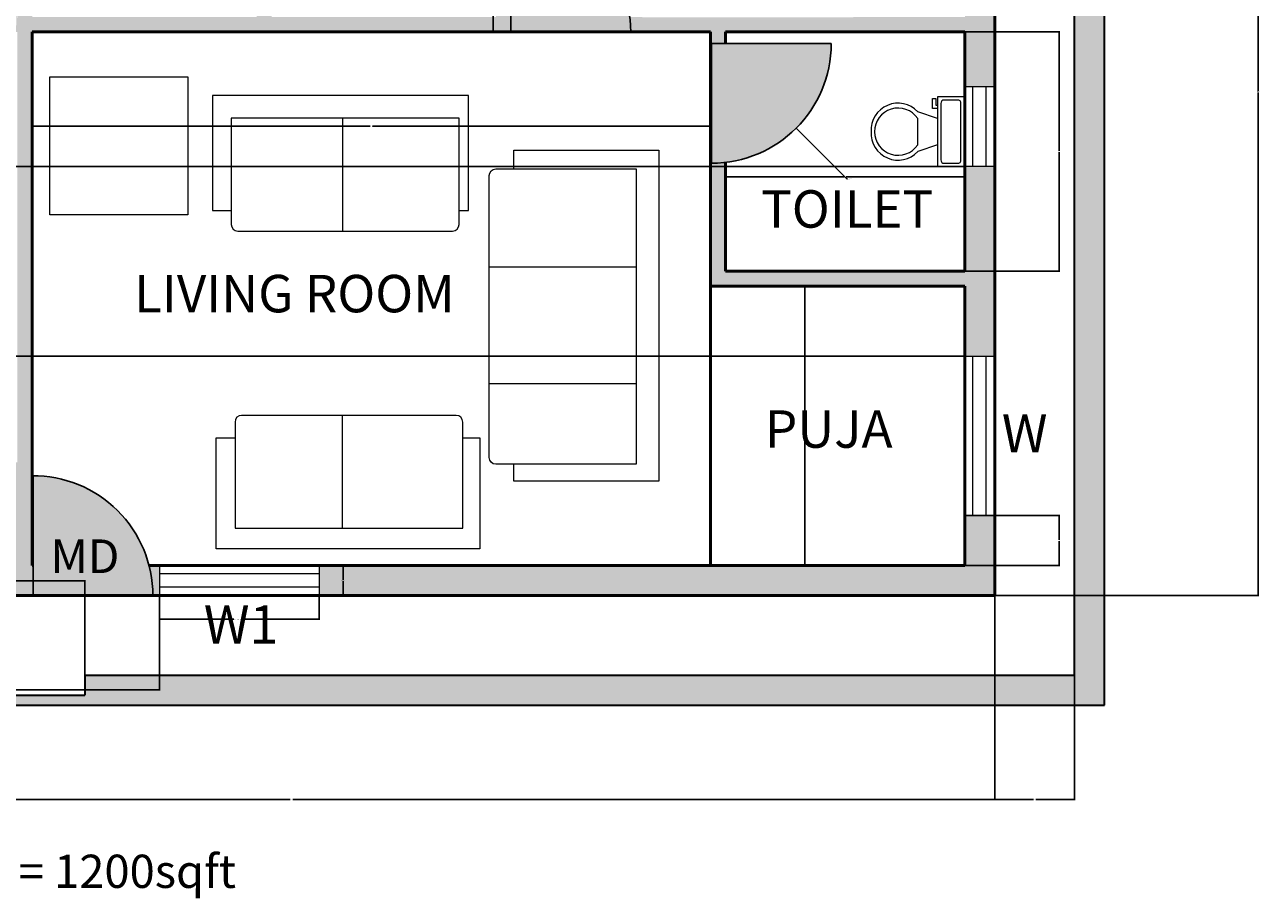
# Model space of a CAD drawing. Units: inches. Extents: x -48 to 546, y -53 to 467.
# Tile 2 of 3: x 174 to 546, y -53 to 210. Entities that reach past the tile are written whole.
import ezdxf

# ---------------------------------------------------------------- set-up
doc = ezdxf.new("R2010")
doc.units = ezdxf.units.IN
doc.header["$MEASUREMENT"] = 0
for name, color, linetype, lineweight in [('A-ANNO-DIMS', 2, 'Continuous', 18), ('A-ANNO-SYMB', 7, 'Continuous', 18), ('A-ANNO-TEXT', 7, 'Continuous', 18), ('A-AREA-IDEN', 7, 'Continuous', 25), ('A-DOOR', 4, 'Continuous', 25), ('A-FLOR-FIXT', 9, 'Continuous', 18), ('A-FURN', 8, 'Continuous', 18), ('A-GLAZ', 4, 'Continuous', 18), ('A-WALL', 7, 'Continuous', 50), ('C-PROP', 7, 'Continuous', 35)]:
    doc.layers.add(name, color=color, linetype=linetype, lineweight=lineweight)
for name, color, linetype, lineweight, true_color in [('A-FLOR-PATT', 253, 'Continuous', 13, 0x9898cc), ('A-WALL-PATT', 251, 'Continuous', 13, 0x636466), ('C-PROP-PATT', 251, 'Continuous', 13, 0x636466)]:
    doc.layers.add(name, color=color, linetype=linetype, lineweight=lineweight, true_color=true_color)
doc.styles.get("Standard").update_dxf_attribs({"font": 'arial.ttf'})
doc.dimstyles.get("Standard").update_dxf_attribs({"dimtxt": 0.18, "dimasz": 0.18, "dimexe": 0.18, "dimexo": 0.0625, "dimgap": 0.09, "dimtad": 0, "dimtih": 1, "dimtoh": 1, "dimdec": 4, "dimzin": 0, "dimdsep": 46, "dimtxsty": 'Standard', "dimcen": 0.09, "dimadec": 0, "dimazin": 0, "dimtfac": 1, "dimtdec": 4, "dimtofl": 0, "dimtmove": 0, "dimatfit": 3, "dimfxl": 1, "dimtolj": 1, "dimtzin": 0, "dimarcsym": 0})
picture_1 = doc.add_image_def('image1.png', size_in_pixel=(1024, 1024))

# ---------------------------------------------------------------- blocks, each defined once
blk = doc.blocks.new('*U2')
for p, q in [((9.5, -6), (9.5, -2)), ((-10, -8.5), (-8, -8.5)), ((-10, -9.5), (-10, -8.5)), ((-7, -9.5), (-10, -9.5)), ((-8, -8.5), (-8, -8)), ((-7, -8), (-7, -9.5)), ((-4, -8), (-6, -14)), ((4, -8), (6, -14)), ((4, -14), (-4, -14))]:
    blk.add_line(p, q)
blk.add_lwpolyline([(10.5, -8), (10.5, 0), (-10.5, 0), (-10.5, -8)], close=True)
for points in [[(-9.5, -2), (-9.5, -6)], [(8.5, -1), (-8.5, -1)], [(-8.5, -7), (8.5, -7)]]:
    blk.add_lwpolyline(points)
for centre, radius, start, end in [((-8.625, -1.875), 0.8839, 81.8699, 188.1301), ((8.625, -1.875), 0.8839, 351.8699, 98.1301), ((-8.625, -6.125), 0.8839, 171.869898, 278.1301), ((8.625, -6.125), 0.8839, 261.8699, 8.1301), ((-0.4772, -19.9188), 8.0953, 133.01722, 273.38), ((0.0374, -19.8731), 7.127, 124.50543, 269.7), ((-0.0373, -19.8731), 7.127, 270.3, 55.4946), ((0.4773, -19.9188), 8.0953, 266.62, 46.9828)]:
    blk.add_arc(centre, radius, start, end)
blk = doc.blocks.new('DOOR-SWING-36IN')
for p, q in [((0, 36), (0, 0)), ((0, 0), (36, 0))]:
    blk.add_line(p, q)
blk.add_arc((0, 0), 36, 0, 90)
blk = doc.blocks.new('VENT-24IN')
for p, q in [((0, 9), (0, 0)), ((24, 9), (24, 0)), ((0, 6.5), (24, 6.5)), ((0, 2.5), (24, 2.5))]:
    blk.add_line(p, q)
blk = doc.blocks.new('WIN-48IN-FRONT')
for p, q in [((0, 9), (0, 0)), ((48, 9), (48, 0)), ((48, 6.49), (0, 6.49)), ((48, 2.49), (0, 2.49)), ((48, 2.49), (0, 2.49)), ((48, 2.49), (0, 2.49))]:
    blk.add_line(p, q)
blk = doc.blocks.new('*D14')
at = {"layer": 'A-ANNO-DIMS', "color": 0, "lineweight": -2, "transparency": 16777216}
for p, q in [((320.64, 244.01), (315.12, 244.01)), ((315.3, 243.83), (315.3, 226.2)), ((315.3, 208.19), (315.3, 225.83)), ((320.64, 208.01), (315.12, 208.01))]:
    blk.add_line(p, q, dxfattribs=at)
at = {"layer": 'A-ANNO-DIMS', "color": 0, "transparency": 16777216}
for points in [[(315.27, 243.83), (315.33, 243.83), (315.3, 244.01)], [(315.27, 208.19), (315.33, 208.19), (315.3, 208.01)]]:
    blk.add_solid(points, dxfattribs=at)
at = {"layer": 'Defpoints', "color": 0, "transparency": 16777216}
for p in [(315.3, 244.01), (320.7, 244.01), (320.7, 208.01)]:
    blk.add_point(p, dxfattribs=at)
at = {"layer": 'A-ANNO-DIMS', "color": 0, "transparency": 16777216, "insert": (315.3, 226.01), "char_height": 0.18, "attachment_point": 5}
blk.add_mtext('\\A1;DOOR 3\'-0" TYP.', dxfattribs=at)
blk = doc.blocks.new('*D18')
at = {"layer": 'A-ANNO-DIMS', "color": 0, "lineweight": -2, "transparency": 16777216}
for p, q in [((215, 38.45), (215, 31.13)), ((263, 38.45), (263, 31.13)), ((215.18, 31.31), (237.31, 31.31)), ((262.82, 31.31), (240.69, 31.31))]:
    blk.add_line(p, q, dxfattribs=at)
at = {"layer": 'A-ANNO-DIMS', "color": 0, "transparency": 16777216}
for points in [[(215.18, 31.34), (215.18, 31.28), (215, 31.31)], [(262.82, 31.34), (262.82, 31.28), (263, 31.31)]]:
    blk.add_solid(points, dxfattribs=at)
at = {"layer": 'Defpoints', "color": 0, "transparency": 16777216}
for p in [(215, 38.51), (263, 38.51), (263, 31.31)]:
    blk.add_point(p, dxfattribs=at)
at = {"layer": 'A-ANNO-DIMS', "color": 0, "transparency": 16777216, "insert": (239, 31.31), "char_height": 0.18, "attachment_point": 5}
blk.add_mtext('\\A1;FRONT WINDOW 4\'-0" TYP.', dxfattribs=at)
blk = doc.blocks.new('*D19')
at = {"layer": 'A-ANNO-DIMS', "color": 0, "lineweight": -2, "transparency": 16777216}
for p, q in [((263.06, 47.51), (270.38, 47.51)), ((270.2, 47.33), (270.2, 43.2)), ((270.2, 38.69), (270.2, 42.83)), ((263.06, 38.51), (270.38, 38.51))]:
    blk.add_line(p, q, dxfattribs=at)
at = {"layer": 'A-ANNO-DIMS', "color": 0, "transparency": 16777216}
for points in [[(270.17, 47.33), (270.23, 47.33), (270.2, 47.51)], [(270.17, 38.69), (270.23, 38.69), (270.2, 38.51)]]:
    blk.add_solid(points, dxfattribs=at)
at = {"layer": 'Defpoints', "color": 0, "transparency": 16777216}
for p in [(263, 47.51), (270.2, 47.51), (263, 38.51)]:
    blk.add_point(p, dxfattribs=at)
at = {"layer": 'A-ANNO-DIMS', "color": 0, "transparency": 16777216, "insert": (270.2, 43.01), "char_height": 0.18, "attachment_point": 5}
blk.add_mtext('\\A1;0\'-9" TYP.', dxfattribs=at)
blk = doc.blocks.new('*D26')
at = {"layer": 'A-ANNO-DIMS', "color": 0, "lineweight": -2, "transparency": 16777216}
for p, q in [((43.2, 38.45), (43.2, -23.08)), ((466.2, 38.45), (466.2, -23.08)), ((43.38, -22.9), (254.3, -22.9)), ((466.02, -22.9), (255.1, -22.9))]:
    blk.add_line(p, q, dxfattribs=at)
at = {"layer": 'A-ANNO-DIMS', "color": 0, "transparency": 16777216}
for points in [[(43.38, -22.87), (43.38, -22.93), (43.2, -22.9)], [(466.02, -22.87), (466.02, -22.93), (466.2, -22.9)]]:
    blk.add_solid(points, dxfattribs=at)
at = {"layer": 'Defpoints', "color": 0, "transparency": 16777216}
for p in [(43.2, 38.51), (466.2, 38.51), (466.2, -22.9)]:
    blk.add_point(p, dxfattribs=at)
at = {"layer": 'A-ANNO-DIMS', "color": 0, "transparency": 16777216, "insert": (254.7, -22.9), "char_height": 0.18, "attachment_point": 5}
blk.add_mtext('\\A1;35\'-3"', dxfattribs=at)
blk = doc.blocks.new('*D27')
at = {"layer": 'A-ANNO-DIMS', "color": 0, "lineweight": -2, "transparency": 16777216}
for p, q in [((466.26, 341.51), (545.59, 341.51)), ((545.41, 341.33), (545.41, 190.2)), ((545.41, 38.69), (545.41, 189.83)), ((466.26, 38.51), (545.59, 38.51))]:
    blk.add_line(p, q, dxfattribs=at)
at = {"layer": 'A-ANNO-DIMS', "color": 0, "transparency": 16777216}
for points in [[(545.38, 341.33), (545.44, 341.33), (545.41, 341.51)], [(545.38, 38.69), (545.44, 38.69), (545.41, 38.51)]]:
    blk.add_solid(points, dxfattribs=at)
at = {"layer": 'Defpoints', "color": 0, "transparency": 16777216}
for p in [(466.2, 341.51), (545.41, 341.51), (466.2, 38.51)]:
    blk.add_point(p, dxfattribs=at)
at = {"layer": 'A-ANNO-DIMS', "color": 0, "transparency": 16777216, "insert": (545.41, 190.01), "char_height": 0.18, "attachment_point": 5}
blk.add_mtext('\\A1;25\'-3"', dxfattribs=at)
blk = doc.blocks.new('*D28')
at = {"layer": 'A-ANNO-DIMS', "color": 0, "lineweight": -2, "transparency": 16777216}
for p, q in [((466.2, 38.45), (466.2, -23.08)), ((490.2, 14.45), (490.2, -23.08)), ((466.38, -22.9), (477.87, -22.9)), ((490.02, -22.9), (478.53, -22.9))]:
    blk.add_line(p, q, dxfattribs=at)
at = {"layer": 'A-ANNO-DIMS', "color": 0, "transparency": 16777216}
for points in [[(466.38, -22.87), (466.38, -22.93), (466.2, -22.9)], [(490.02, -22.87), (490.02, -22.93), (490.2, -22.9)]]:
    blk.add_solid(points, dxfattribs=at)
at = {"layer": 'Defpoints', "color": 0, "transparency": 16777216}
for p in [(466.2, 38.51), (490.2, 14.51), (490.2, -22.9)]:
    blk.add_point(p, dxfattribs=at)
at = {"layer": 'A-ANNO-DIMS', "color": 0, "transparency": 16777216, "insert": (478.2, -22.9), "char_height": 0.18, "attachment_point": 5}
blk.add_mtext('\\A1;2\'-0"', dxfattribs=at)
blk = doc.blocks.new('*D36')
at = {"layer": 'A-ANNO-DIMS', "color": 0, "lineweight": -2, "transparency": 16777216}
for p, q in [((176.7, 207.95), (176.7, 179.43)), ((380.7, 207.95), (380.7, 179.43)), ((176.88, 179.61), (278.31, 179.61)), ((380.52, 179.61), (279.09, 179.61))]:
    blk.add_line(p, q, dxfattribs=at)
at = {"layer": 'A-ANNO-DIMS', "color": 0, "transparency": 16777216}
for points in [[(176.88, 179.64), (176.88, 179.58), (176.7, 179.61)], [(380.52, 179.64), (380.52, 179.58), (380.7, 179.61)]]:
    blk.add_solid(points, dxfattribs=at)
at = {"layer": 'Defpoints', "color": 0, "transparency": 16777216}
for p in [(176.7, 208.01), (380.7, 208.01), (176.7, 179.61)]:
    blk.add_point(p, dxfattribs=at)
at = {"layer": 'A-ANNO-DIMS', "color": 0, "transparency": 16777216, "insert": (278.7, 179.61), "char_height": 0.18, "attachment_point": 5}
blk.add_mtext('\\A1;17\'-0"', dxfattribs=at)
blk = doc.blocks.new('*D37')
at = {"layer": 'A-ANNO-DIMS', "color": 0, "lineweight": -2, "transparency": 16777216}
for p, q in [((385.2, 136.08), (385.2, 164.59)), ((385.38, 164.41), (420.87, 164.41)), ((457.02, 164.41), (421.53, 164.41)), ((457.2, 136.08), (457.2, 164.59))]:
    blk.add_line(p, q, dxfattribs=at)
at = {"layer": 'A-ANNO-DIMS', "color": 0, "transparency": 16777216}
for points in [[(385.38, 164.44), (385.38, 164.38), (385.2, 164.41)], [(457.02, 164.44), (457.02, 164.38), (457.2, 164.41)]]:
    blk.add_solid(points, dxfattribs=at)
at = {"layer": 'Defpoints', "color": 0, "transparency": 16777216}
for p in [(457.2, 164.41), (385.2, 136.01), (457.2, 136.01)]:
    blk.add_point(p, dxfattribs=at)
at = {"layer": 'A-ANNO-DIMS', "color": 0, "transparency": 16777216, "insert": (421.2, 164.41), "char_height": 0.18, "attachment_point": 5}
blk.add_mtext('\\A1;6\'-0"', dxfattribs=at)
blk = doc.blocks.new('*D38')
at = {"layer": 'A-ANNO-DIMS', "color": 0, "lineweight": -2, "transparency": 16777216}
for p, q in [((457.26, 208.01), (485.78, 208.01)), ((485.6, 207.83), (485.6, 172.2)), ((485.6, 136.19), (485.6, 171.83)), ((457.26, 136.01), (485.78, 136.01))]:
    blk.add_line(p, q, dxfattribs=at)
at = {"layer": 'A-ANNO-DIMS', "color": 0, "transparency": 16777216}
for points in [[(485.57, 207.83), (485.63, 207.83), (485.6, 208.01)], [(485.57, 136.19), (485.63, 136.19), (485.6, 136.01)]]:
    blk.add_solid(points, dxfattribs=at)
at = {"layer": 'Defpoints', "color": 0, "transparency": 16777216}
for p in [(457.2, 208.01), (457.2, 136.01), (485.6, 136.01)]:
    blk.add_point(p, dxfattribs=at)
at = {"layer": 'A-ANNO-DIMS', "color": 0, "transparency": 16777216, "insert": (485.6, 172.01), "char_height": 0.18, "attachment_point": 5}
blk.add_mtext('\\A1;6\'-0"', dxfattribs=at)
blk = doc.blocks.new('*D39')
at = {"layer": 'A-ANNO-DIMS', "color": 0, "lineweight": -2, "transparency": 16777216}
for p, q in [((380.76, 131.51), (409.28, 131.51)), ((409.1, 131.33), (409.1, 89.7)), ((409.1, 47.69), (409.1, 89.33)), ((380.76, 47.51), (409.28, 47.51))]:
    blk.add_line(p, q, dxfattribs=at)
at = {"layer": 'A-ANNO-DIMS', "color": 0, "transparency": 16777216}
for points in [[(409.07, 131.33), (409.13, 131.33), (409.1, 131.51)], [(409.07, 47.69), (409.13, 47.69), (409.1, 47.51)]]:
    blk.add_solid(points, dxfattribs=at)
at = {"layer": 'Defpoints', "color": 0, "transparency": 16777216}
for p in [(380.7, 131.51), (380.7, 47.51), (409.1, 47.51)]:
    blk.add_point(p, dxfattribs=at)
at = {"layer": 'A-ANNO-DIMS', "color": 0, "transparency": 16777216, "insert": (409.1, 89.51), "char_height": 0.18, "attachment_point": 5}
blk.add_mtext('\\A1;7\'-0"', dxfattribs=at)
blk = doc.blocks.new('*D41')
at = {"layer": 'A-ANNO-DIMS', "color": 0, "lineweight": -2, "transparency": 16777216}
for p, q in [((120, 38.45), (120, 9.93)), ((215, 38.45), (215, 9.93)), ((120.18, 10.11), (167.1, 10.11)), ((214.82, 10.11), (167.9, 10.11))]:
    blk.add_line(p, q, dxfattribs=at)
at = {"layer": 'A-ANNO-DIMS', "color": 0, "transparency": 16777216}
for points in [[(120.18, 10.14), (120.18, 10.08), (120, 10.11)], [(214.82, 10.14), (214.82, 10.08), (215, 10.11)]]:
    blk.add_solid(points, dxfattribs=at)
at = {"layer": 'Defpoints', "color": 0, "transparency": 16777216}
for p in [(120, 38.51), (215, 38.51), (120, 10.11)]:
    blk.add_point(p, dxfattribs=at)
at = {"layer": 'A-ANNO-DIMS', "color": 0, "transparency": 16777216, "insert": (167.5, 10.11), "char_height": 0.18, "attachment_point": 5}
blk.add_mtext('\\A1;7\'-11"', dxfattribs=at)
blk = doc.blocks.new('*D44')
at = {"layer": 'A-ANNO-DIMS', "color": 0, "lineweight": -2, "transparency": 16777216}
for p, q in [((457.26, 62.5), (485.78, 62.5)), ((485.6, 62.32), (485.6, 55.19)), ((485.6, 47.69), (485.6, 54.82)), ((457.26, 47.51), (485.78, 47.51))]:
    blk.add_line(p, q, dxfattribs=at)
at = {"layer": 'A-ANNO-DIMS', "color": 0, "transparency": 16777216}
for points in [[(485.57, 62.32), (485.63, 62.32), (485.6, 62.5)], [(485.57, 47.69), (485.63, 47.69), (485.6, 47.51)]]:
    blk.add_solid(points, dxfattribs=at)
at = {"layer": 'Defpoints', "color": 0, "transparency": 16777216}
for p in [(457.2, 62.5), (457.2, 47.51), (485.6, 47.51)]:
    blk.add_point(p, dxfattribs=at)
at = {"layer": 'A-ANNO-DIMS', "color": 0, "transparency": 16777216, "insert": (485.6, 55.01), "char_height": 0.18, "attachment_point": 5}
blk.add_mtext('\\A1;1\'-3"', dxfattribs=at)
blk = doc.blocks.new('*D45')
at = {"layer": 'A-ANNO-DIMS', "color": 0, "lineweight": -2, "transparency": 16777216}
for p, q in [((456.95, 167.5), (-18.38, 167.5)), ((-18.2, 167.32), (-18.2, 139.18)), ((-18.2, 110.68), (-18.2, 138.82)), ((457.14, 110.5), (-18.38, 110.5))]:
    blk.add_line(p, q, dxfattribs=at)
at = {"layer": 'A-ANNO-DIMS', "color": 0, "transparency": 16777216}
for points in [[(-18.23, 167.32), (-18.17, 167.32), (-18.2, 167.5)], [(-18.23, 110.68), (-18.17, 110.68), (-18.2, 110.5)]]:
    blk.add_solid(points, dxfattribs=at)
at = {"layer": 'Defpoints', "color": 0, "transparency": 16777216}
for p in [(457.01, 167.5), (-18.2, 110.5), (457.2, 110.5)]:
    blk.add_point(p, dxfattribs=at)
at = {"layer": 'A-ANNO-DIMS', "color": 0, "transparency": 16777216, "insert": (-18.2, 139), "char_height": 0.18, "attachment_point": 5}
blk.add_mtext('\\A1;4\'-9"', dxfattribs=at)
blk = doc.blocks.new('*D49')
at = {"layer": 'A-ANNO-DIMS', "color": 0, "lineweight": -2, "transparency": 16777216}
for p, q in [((103, 14.58), (103, 43.09)), ((103.18, 42.91), (147.21, 42.91)), ((192.32, 42.91), (148.29, 42.91)), ((192.5, 14.58), (192.5, 43.09))]:
    blk.add_line(p, q, dxfattribs=at)
at = {"layer": 'A-ANNO-DIMS', "color": 0, "transparency": 16777216}
for points in [[(103.18, 42.94), (103.18, 42.88), (103, 42.91)], [(192.32, 42.94), (192.32, 42.88), (192.5, 42.91)]]:
    blk.add_solid(points, dxfattribs=at)
at = {"layer": 'Defpoints', "color": 0, "transparency": 16777216}
for p in [(192.5, 42.91), (103, 14.51), (192.5, 14.51)]:
    blk.add_point(p, dxfattribs=at)
at = {"layer": 'A-ANNO-DIMS', "color": 0, "transparency": 16777216, "insert": (147.75, 42.91), "char_height": 0.18, "attachment_point": 5}
blk.add_mtext('\\A1;7\'-5 1/2"', dxfattribs=at)
blk = doc.blocks.new('*D51')
at = {"layer": 'A-ANNO-DIMS', "color": 0, "lineweight": -2, "transparency": 16777216}
for p, q in [((380.91, 204.5), (381.09, 204.5)), ((381, 204.41), (381, 204.59)), ((421.73, 163.77), (406.58, 178.92)), ((421.91, 163.77), (421.73, 163.77))]:
    blk.add_line(p, q, dxfattribs=at)
at = {"layer": 'A-ANNO-DIMS', "color": 0, "transparency": 16777216}
blk.add_solid([(406.6, 178.94), (406.56, 178.9), (406.46, 179.04)], dxfattribs=at)
at = {"layer": 'Defpoints', "color": 0, "transparency": 16777216}
for p in [(381, 204.5), (406.46, 179.04)]:
    blk.add_point(p, dxfattribs=at)
at = {"layer": 'A-ANNO-DIMS', "color": 0, "transparency": 16777216, "insert": (422.52, 163.77), "char_height": 0.18, "attachment_point": 5}
blk.add_mtext('\\A1;6X R3\'-0"', dxfattribs=at)

msp = doc.modelspace()

# ---------------------------------------------------------------- hatches: boundary and pattern name
at = {"layer": 'A-FLOR-PATT'}
h = msp.add_hatch(color=256, dxfattribs=at)
h.dxf.hatch_style = 1
h.paths.add_polyline_path([(208.19994, 330.01344), (172.19994, 330.01344), (172.19994, 294.01344, 0.414213549)])
h.paths.add_polyline_path([(320.5, 332.5), (284.5, 332.5, 0.414213562), (320.5, 296.5)])
h.paths.add_polyline_path([(417, 204.5), (381, 204.5), (381, 168.5, 0.414213562)])
h.paths.add_polyline_path([(177, 74.5), (177, 38.51344), (213, 38.51344, 0.414104244)])
h.paths.add_polyline_path([(172, 244, 0.414104258), (136, 208.01344), (172, 208.01344)])
h.paths.add_polyline_path([(320.69994, 244.01344), (320.69994, 212.51344), (320.69994, 208.01344), (356.69994, 208.01344, 0.414213532)])
h.paths.add_polyline_path([(172.19994, 78.5), (52.19994, 78.5), (52.19994, 47.51344), (172.19994, 47.51344)])
h.paths.add_polyline_path([(126, 74), (166, 74), (166, 54.5), (126, 54.5)], flags=16)
h.paths.add_polyline_path([(101, 53), (56.5, 53), (56.5, 74.5), (101, 74.5)], flags=16)
h.paths.add_polyline_path([(141, 69), (162.5, 69), (162.5, 58.5), (141, 58.5)], flags=0)
h.paths.add_polyline_path([(97.5, 55), (83, 55), (83, 67.5), (97.5, 67.5)], flags=0)
h.paths.add_polyline_path([(84, 61.5, -1), (96, 61.5, -1)], flags=0)
h.paths.add_polyline_path([(88.5, 71.5, -1), (92.5, 71.5, -1)], flags=0)
h.paths.add_polyline_path([(90, 71.5, -1), (91, 71.5, -1)], flags=0)
h.paths.add_polyline_path([(162, 64.5, -1), (158, 64.5, -1)], flags=0)
h.paths.add_polyline_path([(75, 55), (60.5, 55), (60.5, 67.5), (75, 67.5)], flags=0)
h.paths.add_polyline_path([(61.5, 61.5, -1), (73.5, 61.5, -1)], flags=0)
h.paths.add_polyline_path([(66, 71.5, -1), (70, 71.5, -1)], flags=0)
h.paths.add_polyline_path([(67.5, 71.5, -1), (68.5, 71.5, -1)], flags=0)
h.paths.add_polyline_path([(176.42827, 40.63764), (207.16292, 40.63764), (207.16292, 57.88764), (176.42827, 57.88764)], flags=9)
h = msp.add_hatch(color=256, dxfattribs=at)
h.dxf.hatch_style = 1
h.paths.add_polyline_path([(177, 74.5), (177, 38.51344), (213, 38.51344, 0.414104244)])
at = {"layer": 'A-WALL-PATT'}
h = msp.add_hatch(color=256, dxfattribs=at)
h.dxf.hatch_style = 1
h.paths.add_polyline_path([(282.44994, 341.51344), (234.44994, 341.51344), (234.44994, 332.51344), (244.19994, 332.51344), (244.19994, 212.51344), (176.69994, 212.51344), (176.69994, 294.29579, -0.031342215), (172.19994, 294.01344), (172.19994, 212.51344), (172.00059, 208.01344), (172.19994, 208.01344), (172.19994, 47.51344), (120, 47.51344), (120, 38.51344), (177, 38.51344), (177, 47.51344), (176.69994, 47.51344), (176.69994, 208.01344), (320.69994, 208.01344), (320.69994, 244.01344), (320.69994, 296.50056, -0.031331714), (316.19994, 296.75774), (316.19994, 212.51344), (248.69994, 212.51344), (248.69994, 332.51344), (282.44994, 332.51344)])
h.paths.add_polyline_path([(466.19994, 341.51344), (306.44994, 341.51344), (306.44994, 332.51344), (316.19994, 332.51344), (457.19994, 332.51344), (457.19994, 304.5), (466.19994, 304.5)])
h.paths.add_polyline_path([(466.19994, 256.5), (457.19994, 256.5), (457.19994, 212.51344), (423.64319, 212.51344), (423.64319, 212.34928), (365.34701, 212.34928), (356.41758, 212.51344, -0.031342215), (356.69994, 208.01344), (380.69994, 208.01344), (380.69994, 204.5), (385.19994, 204.5), (385.19994, 208.01344), (457.19994, 208.01344), (457.19994, 191.5), (466.19994, 191.5)])
h.paths.add_polyline_path([(210.44994, 341.51344), (43.19994, 341.51344), (43.19994, 303.5), (52.19994, 303.5), (52.19994, 332.51344), (172.19994, 332.51344), (172.19994, 330.01344), (176.69994, 330.01344), (176.69994, 332.51344), (210.44994, 332.51344)])
h.paths.add_polyline_path([(52.19994, 208.01344), (136, 208.01344, -0.031342955), (136.28405, 212.51344), (52.19994, 212.51344), (52.19994, 255.5), (43.19994, 255.5), (43.19994, 38.51344), (72, 38.51344), (72, 47.51344), (52.19994, 47.51344)])
h.paths.add_polyline_path([(466.19994, 62.5), (457.19994, 62.5), (457.19994, 47.51344), (380.69994, 47.51344), (263, 47.51344), (263, 38.51344), (466.19994, 38.51344)])
h.paths.add_polyline_path([(215, 47.51344), (211.85338, 47.51344, -0.063257301), (213, 38.51344), (215, 38.51344)])
h.paths.add_polyline_path([(466.19994, 167.5), (457.19994, 167.5), (457.19994, 136.01344), (385.19994, 136.01344), (385.19994, 168.74583, -0.031326837), (380.69994, 168.50125), (380.69994, 131.51344), (457.19994, 131.51344), (457.19994, 110.5), (466.19994, 110.5)])
h = msp.add_hatch(color=256, dxfattribs=at)
h.dxf.hatch_style = 1
h.paths.add_polyline_path([(210.44994, 341.51344), (43.19994, 341.51344), (43.19994, 303.5), (52.19994, 303.5), (52.19994, 332.51344), (172.19994, 332.51344), (172.19994, 330.01344), (176.69994, 330.01344), (176.69994, 332.51344), (210.44994, 332.51344)])
h.paths.add_polyline_path([(466.19994, 341.51344), (306.44994, 341.51344), (306.44994, 332.51344), (316.19994, 332.51344), (457.19994, 332.51344), (457.19994, 304.5), (466.19994, 304.5)])
h.paths.add_polyline_path([(282.44994, 341.51344), (234.44994, 341.51344), (234.44994, 332.51344), (244.19994, 332.51344), (244.19994, 212.51344), (176.69994, 212.51344), (176.69994, 294.29579, -0.031342215), (172.19994, 294.01344), (172.19994, 212.51344), (172.00059, 208.01344), (172.19994, 208.01344), (172.19994, 47.51344), (120, 47.51344), (120, 38.51344), (177, 38.51344), (177, 47.51344), (176.69994, 47.51344), (176.69994, 208.01344), (320.69994, 208.01344), (320.69994, 244.01344), (320.69994, 296.50056, -0.031331714), (316.19994, 296.75774), (316.19994, 212.51344), (248.69994, 212.51344), (248.69994, 332.51344), (282.44994, 332.51344)])
h.paths.add_polyline_path([(52.19994, 255.5), (43.19994, 255.5), (43.19994, 38.51344), (72, 38.51344), (72, 47.51344), (52.19994, 47.51344), (52.19994, 208.01344), (136, 208.01344, -0.031342955), (136.28405, 212.51344), (52.19994, 212.51344)])
h.paths.add_polyline_path([(466.19994, 256.5), (457.19994, 256.5), (457.19994, 212.51344), (423.64319, 212.51344), (423.64319, 212.34928), (365.34701, 212.34928), (356.41758, 212.51344, -0.031342215), (356.69994, 208.01344), (380.69994, 208.01344), (380.69994, 204.5), (385.19994, 204.5), (385.19994, 208.01344), (457.19994, 208.01344), (457.19994, 191.5), (466.19994, 191.5)])
h.paths.add_polyline_path([(466.19994, 167.5), (457.19994, 167.5), (457.19994, 136.01344), (385.19994, 136.01344), (385.19994, 168.74583, -0.031326837), (380.69994, 168.50125), (380.69994, 131.51344), (457.19994, 131.51344), (457.19994, 110.5), (466.19994, 110.5)])
h.paths.add_polyline_path([(466.19994, 62.5), (457.19994, 62.5), (457.19994, 47.51344), (380.69994, 47.51344), (263, 47.51344), (263, 38.51344), (466.19994, 38.51344)])
h.paths.add_polyline_path([(215, 47.51344), (211.85338, 47.51344, -0.063257301), (213, 38.51344), (215, 38.51344)])
at = {"layer": 'C-PROP-PATT'}
h = msp.add_hatch(color=256, dxfattribs=at)
h.dxf.hatch_style = 1
h.paths.add_polyline_path([(499.19994, 374.51344), (10.19994, 374.51344), (10.19994, 5.51344), (103, 5.51344), (103, 14.51344), (19.19994, 14.51344), (19.19994, 365.51344), (490.19994, 365.51344), (490.19994, 14.51344), (192.5, 14.51344), (192.5, 5.51344), (499.19994, 5.51344)])
h = msp.add_hatch(color=256, dxfattribs=at)
h.dxf.hatch_style = 1
h.paths.add_polyline_path([(192.5, 8.5), (103, 8.5), (103, 5.5), (192.5, 5.5)])

# ---------------------------------------------------------------- linework, layer by layer
at = {"layer": 'A-DOOR'}
for p, q in [((417, 204.5), (380.69994, 204.5)), ((381, 204.5), (381, 168.5)), ((177, 74.5), (177, 38.5)), ((177, 38.5), (213, 38.5))]:
    msp.add_line(p, q, dxfattribs=at)
for centre, start, end in [((381, 204.5), 270, 0), ((177, 38.5), 0, 90.4775597)]:
    msp.add_arc(centre, 36, start, end, dxfattribs=at)
at = {"layer": 'A-FURN'}
for p, q in [((269.97917, 182.0553), (269.97917, 148.07718)), ((314.08115, 137.36171), (358.24372, 137.36171)), ((314.08115, 102.29131), (358.24372, 102.29131)), ((269.97455, 92.72533), (269.97455, 58.6555))]:
    msp.add_line(p, q, dxfattribs=at)
for points in [[(305.09029, 154.33241), (307.92183, 154.33241), (307.92183, 188.84458), (230.9039, 188.84458), (230.9039, 154.33241), (236.56698, 154.33241)], [(321.51323, 166.77943), (321.51323, 172.43716), (365.11896, 172.43716), (365.11896, 72.86107), (321.51323, 72.86107), (321.51323, 77.95303)], [(306.2229, 85.87385), (311.31968, 85.87385), (311.31968, 52.49324), (232.03652, 52.49324), (232.03652, 85.87385), (237.6996, 85.87385)]]:
    msp.add_lwpolyline(points, dxfattribs=at)
for points in [[(238.56698, 148.10891), (303.09029, 148.10891, 0.414213562), (305.09029, 150.10891), (305.09029, 182.0553), (236.56698, 182.0553), (236.56698, 150.10891, 0.414213562)], [(316.15122, 166.77943), (358.32326, 166.77943), (358.32326, 77.95303), (316.15122, 77.95303, -0.414213562), (314.15122, 79.95303), (314.15122, 164.77943, -0.414213562)], [(237.6996, 58.71674), (306.2229, 58.71674), (306.2229, 90.66313, 0.414213562), (304.2229, 92.66313), (239.6996, 92.66313, 0.414213562), (237.6996, 90.66313)]]:
    msp.add_lwpolyline(points, format="xyb", close=True, dxfattribs=at)
at = {"layer": 'A-GLAZ'}
for p, q in [((457.19994, 110.5), (466.19994, 110.5)), ((459.50001, 110.5), (459.50001, 62.5)), ((463.50001, 110.5), (463.50001, 62.5)), ((463.50001, 110.5), (463.50001, 62.5)), ((463.50001, 110.5), (463.50001, 62.5)), ((457.19994, 62.5), (466.19994, 62.5))]:
    msp.add_line(p, q, dxfattribs=at)
at = {"layer": 'A-WALL'}
for p, q in [((466.19994, 38.51344), (466.19994, 341.51344)), ((176.69994, 47.51344), (176.69994, 208.01344)), ((176.69994, 208.01344), (380.69994, 208.01344)), ((380.69994, 47.51344), (380.69994, 208.01344)), ((385.19994, 208.01344), (457.19994, 208.01344)), ((385.19994, 204.5), (385.19994, 208.01344)), ((457.19994, 136.01344), (457.19994, 208.01344)), ((385.19994, 136.01344), (385.19994, 168.74583)), ((385.19994, 136.01344), (457.19994, 136.01344)), ((380.69994, 131.51344), (457.19994, 131.51344)), ((457.19994, 47.51344), (457.19994, 131.51344)), ((176.69994, 47.51344), (177, 47.51344)), ((211.85338, 47.51344), (380.69994, 47.51344)), ((380.69994, 47.51344), (457.19994, 47.51344)), ((43.19994, 38.51344), (466.19994, 38.51344))]:
    msp.add_line(p, q, dxfattribs=at)
at = {"layer": 'C-PROP'}
for p, q in [((499.19994, 5.51344), (499.19994, 374.51344)), ((490.19994, 14.51344), (490.19994, 365.51344)), ((192.5, 14.51344), (490.19994, 14.51344)), ((103, 8.5), (192.5, 8.5)), ((103, 5.5), (192.5, 5.5)), ((192.5, 5.51344), (499.19994, 5.51344))]:
    msp.add_line(p, q, dxfattribs=at)
for points in [[(192.5, 14.51344), (192.5, 8.5)], [(192.5, 5.51344), (192.5, 5.5)]]:
    msp.add_lwpolyline(points, dxfattribs=at)

# ---------------------------------------------------------------- block references
at = {"layer": 'A-DOOR'}
msp.add_blockref('DOOR-SWING-36IN', (320.7, 208.013), dxfattribs=at)
at = {"layer": 'A-FLOR-FIXT', "rotation": 270}
msp.add_blockref('*U2', (457.01404, 178), dxfattribs=at)
at = {"layer": 'A-GLAZ', "rotation": 269.9999999999997}
msp.add_blockref('VENT-24IN', (457.01361, 191.49994), dxfattribs=at)
at = {"layer": 'A-GLAZ'}
msp.add_blockref('WIN-48IN-FRONT', (215, 38.513), dxfattribs=at)

# ---------------------------------------------------------------- texts
at = {"layer": 'A-ANNO-TEXT'}
for s, height, p in [('W', 11.5, (468.30327, 81.51264)), ('MD', 10.126217, (182.21474, 45.22099)), ('W1', 11.5, (228.30327, 24.01264)), ('TOTAL BUILD UP AREA = 1200sqft', 10, (26.91088, -49.49293))]:
    msp.add_text(s, height=height, dxfattribs=at).set_placement(p)
at = {"layer": 'A-AREA-IDEN'}
for s, height, p in [('TOILET', 11.2677, (395.94878, 149.1085)), ('LIVING ROOM', 11.2676997, (207.36813, 123.6487)), ('PUJA', 11.2677, (397.08139, 82.91303))]:
    msp.add_text(s, height=height, dxfattribs=at).set_placement(p)

# ---------------------------------------------------------------- dimensions: what is measured, and where the dimension line sits
at = {"layer": 'A-ANNO-DIMS'}
for base, p1, p2, angle, picture, middle in [((545.41404, 341.51344), (466.19994, 38.51344), (466.19994, 341.51344), 90, '*D27', (545.41404, 190.01344)), ((176.69994, 179.61344), (380.69994, 208.01344), (176.69994, 208.01344), 180, '*D36', (278.69994, 179.61344)), ((485.59994, 136.01344), (457.19994, 208.01344), (457.19994, 136.01344), 270, '*D38', (485.59994, 172.01344)), ((-18.20006, 110.5), (457.01404, 167.5), (457.19994, 110.5), 90, '*D45', (-18.20006, 139)), ((409.09994, 47.51344), (380.69994, 131.51344), (380.69994, 47.51344), 270, '*D39', (409.09994, 89.51344)), ((485.59994, 47.51344), (457.19994, 62.5), (457.19994, 47.51344), 270, '*D44', (485.59994, 55.00672)), ((120, 10.11344), (215, 38.51344), (120, 38.51344), 180, '*D41', (167.5, 10.11344))]:
    dim = msp.add_linear_dim(base=base, p1=p1, p2=p2, angle=angle, dimstyle='Standard', override={"dimdec": 1, "dimlfac": 1, "dimrnd": 0, "dimzin": 1, "dimdsep": 46, "dimlunit": 4, "dimfrac": 2}, dxfattribs=at)
    dim.commit()
    dim.dimension.update_dxf_attribs({"geometry": picture, "text_midpoint": middle})
for base, p1, p2, text, picture, middle in [((315.29994, 244.01344), (320.69994, 208.01344), (320.69994, 244.01344), 'DOOR <> TYP.', '*D14', (315.29994, 226.01344)), ((270.2, 47.51344), (263, 38.51344), (263, 47.51344), '<> TYP.', '*D19', (270.2, 43.01344))]:
    dim = msp.add_linear_dim(base=base, p1=p1, p2=p2, angle=90, text=text, dimstyle='Standard', override={"dimdec": 1, "dimlfac": 1, "dimrnd": 0, "dimzin": 1, "dimdsep": 46, "dimlunit": 4, "dimfrac": 2}, dxfattribs=at)
    dim.commit()
    dim.dimension.update_dxf_attribs({"geometry": picture, "text_midpoint": middle})
dim = msp.add_radius_dim(center=(381, 204.5), mpoint=(406.45584, 179.04416), text='6X <>', dimstyle='Standard', override={"dimdec": 1, "dimlfac": 1, "dimrnd": 0, "dimzin": 1, "dimdsep": 46, "dimlunit": 4, "dimfrac": 2}, dxfattribs=at)
dim.commit()
dim.dimension.update_dxf_attribs({"geometry": '*D51', "text_midpoint": (422.5186, 163.77065), "dimtype": 164})
for base, p1, p2, picture, middle in [((457.19994, 164.41344), (385.19994, 136.01344), (457.19994, 136.01344), '*D37', (421.19994, 164.41344)), ((192.5, 42.91344), (103, 14.51344), (192.5, 14.51344), '*D49', (147.75, 42.91344)), ((466.19994, -22.9), (43.19994, 38.51344), (466.19994, 38.51344), '*D26', (254.69994, -22.9)), ((490.19994, -22.9), (466.19994, 38.51344), (490.19994, 14.51344), '*D28', (478.19994, -22.9))]:
    dim = msp.add_linear_dim(base=base, p1=p1, p2=p2, dimstyle='Standard', override={"dimdec": 1, "dimlfac": 1, "dimrnd": 0, "dimzin": 1, "dimdsep": 46, "dimlunit": 4, "dimfrac": 2}, dxfattribs=at)
    dim.commit()
    dim.dimension.update_dxf_attribs({"geometry": picture, "text_midpoint": middle})
dim = msp.add_linear_dim(base=(263, 31.31344), p1=(215, 38.51344), p2=(263, 38.51344), text='FRONT WINDOW <> TYP.', dimstyle='Standard', override={"dimdec": 1, "dimlfac": 1, "dimrnd": 0, "dimzin": 1, "dimdsep": 46, "dimlunit": 4, "dimfrac": 2}, dxfattribs=at)
dim.commit()
dim.dimension.update_dxf_attribs({"geometry": '*D18', "text_midpoint": (239, 31.31344)})

# ---------------------------------------------------------------- pictures from other files: only their frames are drawn
at = {"layer": 'A-ANNO-SYMB'}
image = msp.add_image(picture_1, insert=(182, 153), size_in_units=(41.5, 41.5), dxfattribs=at)
image.dxf.flags = 7

doc.saveas('drawing.dxf')
